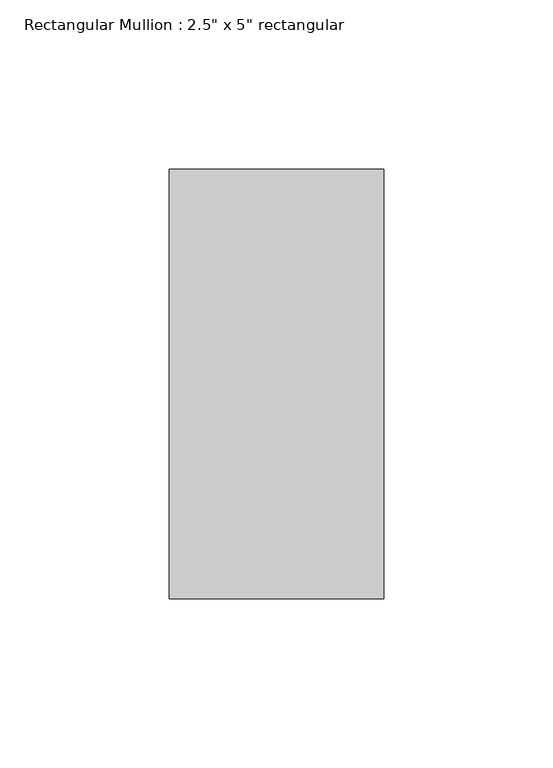
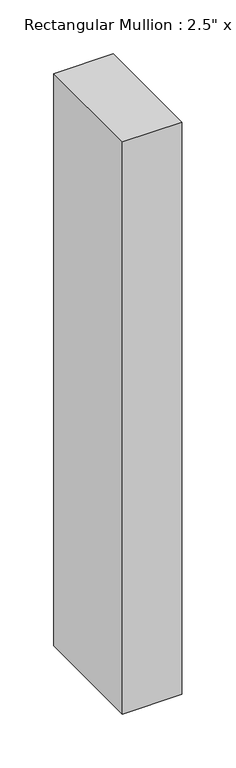
"""IFC4 building model written with IfcOpenShell, lengths in millimetres: member geometry."""

from ifc_helpers import new_model, si_unit, frame, origin, place, context, project, spatial, polyline, outline, extrude, source, transform, mapped, element, save


def member_e53b78c9(model_context):
    return source(origin(), model_context, "Body", "SweptSolid", [
        extrude(outline(polyline([(31.75, 63.5), (31.75, -63.5), (-31.75, -63.5), (-31.75, 63.5), (31.75, 63.5)])), frame((0.0, 0.0, -647.7), z_axis=(0.0, 0.0, 1.0), x_axis=(1.0, 0.0, 0.0)), (0.0, 0.0, 1.0), 647.7),
    ])


if __name__ == "__main__":
    model = new_model("IFC4")
    model_context = context("Model", 3, world=origin())
    ifc_project = project(units=[si_unit("LENGTHUNIT", "METRE", prefix="MILLI")], contexts=[model_context])
    site = spatial("IfcSite", under=ifc_project)
    building = spatial("IfcBuilding", under=site)
    placement = place(None, origin())
    member_shape = member_e53b78c9(model_context)
    element("IfcMember", 1, ObjectType="Rectangular Mullion : 2.5\" x 5\" rectangular", at=placement, inside=building, context=model_context, shape_type="MappedRepresentation", body=[
        mapped(member_shape, transform((0.0, 0.0, 0.0), x_axis=(1.0, 0.0, 0.0), y_axis=(0.0, 1.0, 0.0), z_axis=(0.0, 0.0, 1.0))),
    ])
    save(model, "model.ifc")

# Revit data of these elements
# Type "Rectangular Mullion : 2.5\" x 5\" rectangular"
#   built-in parameter 1007304 = 0.416667 (stored number, unit not read)
#   built-in parameter 1007301 = 0.104167 (stored number, unit not read)
#   built-in parameter 1007300 = 0.104167 (stored number, unit not read)
# Element 1 (IfcMember, "Rectangular Mullion : 2.5\" x 5\" rectangular")
#   Materials on its faces: "Aluminum"
# Materials
#   "Aluminum": class "Metal", colour RGB 247 247 247, transparency 0, Description = "Aluminum 6061", Cost = 0
